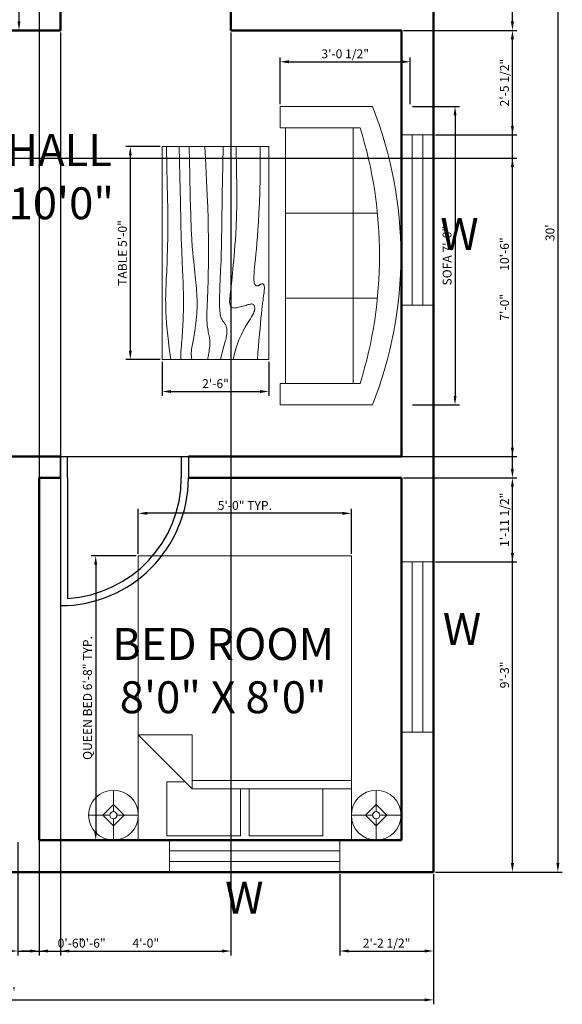
# Model space of a CAD drawing. Units: inches. Extents: x 2530 to 2846, y 1711 to 2145.
# Tile 2 of 3: x 2693 to 2846, y 1711 to 1989. Entities that reach past the tile are written whole.
import ezdxf

# ---------------------------------------------------------------- set-up
doc = ezdxf.new("R2010")
doc.units = ezdxf.units.IN
for name, color, linetype, lineweight in [('A-ANNO-DIMS', 2, 'Continuous', 18), ('A-ANNO-TEXT', 7, 'Continuous', 18), ('A-AREA-IDEN', 7, 'Continuous', 25), ('A-DOOR', 3, 'Continuous', 25), ('A-FURN', 8, 'Continuous', 18), ('A-GLAZ', 4, 'Continuous', 18), ('A-WALL', 7, 'Continuous', 50)]:
    doc.layers.add(name, color=color, linetype=linetype, lineweight=lineweight)
doc.styles.get("Standard").update_dxf_attribs({"font": 'arial.ttf'})
doc.dimstyles.new('ISO-25', dxfattribs={"dimtxt": 2.5, "dimasz": 2.5, "dimexe": 1.25, "dimexo": 0.625, "dimtad": 1, "dimdec": 0, "dimlunit": 3, "dimtxsty": 'Standard', "dimcen": 2.5, "dimadec": 0, "dimazin": 0, "dimtfac": 1, "dimtdec": 0, "dimtmove": 0, "dimatfit": 3, "dimfxl": 1, "dimarcsym": 0})

# ---------------------------------------------------------------- blocks, each defined once
blk = doc.blocks.new('Sofa - Roundback 7 ft.')
for p, q in [((-12.00002, -32.4421), (-12.00003, -6.5971)), ((11.99997, -32.4421), (11.99998, -6.5971)), ((-36.000027, -34), (-36.000027, -11.4696)), ((-35.999844, -13.3819), (35.9998, -13.3819)), ((35.99998, -34), (35.99998, -11.4696)), ((-36.000027, -32.4421), (35.99998, -32.4421))]:
    blk.add_line(p, q)
for points in [[(-36.000027, -34), (-42.000027, -34), (-42.000027, -8)], [(41.99998, -8), (41.99998, -34), (35.99998, -34)]]:
    blk.add_lwpolyline(points)
for centre, radius, start, end in [((0, -114.25), 114.25, 68.43141, 111.5686), ((-0.00001, -127.1968), 121.1968, 72.72033, 107.2797)]:
    blk.add_arc(centre, radius, start, end)
blk = doc.blocks.new('Table - Rectangular Woodgrain 60 x 30 in.')
for p, q in [((0, 0), (0, -30)), ((60, 0), (0, 0)), ((60, -30), (60, 0)), ((0, -30), (60, -30))]:
    blk.add_line(p, q)
for points in [[(0, -2.4), (4.8155, -2.418), (9.0302, -2.4688), (12.709, -2.5477), (15.9167, -2.65), (18.7181, -2.7711), (21.1781, -2.9063), (23.3616, -3.0508), (25.3333, -3.2), (27.1477, -3.3495), (28.8172, -3.4958), (30.3437, -3.636), (31.7291, -3.7667), (32.9756, -3.8849), (34.0849, -3.9875), (35.059, -4.0714), (35.9, -4.1334), (36.6114, -4.1711), (37.2041, -4.1854), (37.6906, -4.1779), (38.0833, -4.15), (38.3948, -4.1034), (38.6375, -4.0396), (38.8239, -3.9602), (38.9666, -3.8667), (39.0764, -3.7608), (39.1573, -3.6448), (39.2116, -3.521), (39.2416, -3.3917), (39.2498, -3.2593), (39.2385, -3.1261), (39.21, -2.9944), (39.1666, -2.8667), (39.111, -2.7447), (39.0468, -2.6281), (38.978, -2.5163), (38.9083, -2.4083), (38.8418, -2.3035), (38.7823, -2.201), (38.7337, -2.1001), (38.7, -2), (38.6844, -1.9003), (38.6875, -1.8021), (38.7094, -1.707), (38.75, -1.6167), (38.8094, -1.5326), (38.8875, -1.4563), (38.9844, -1.3893), (39.1, -1.3333), (39.2351, -1.2896), (39.3937, -1.2583), (39.5804, -1.2396), (39.8, -1.2333), (40.057, -1.2396), (40.3562, -1.2583), (40.7023, -1.2896), (41.1, -1.3333), (41.5547, -1.3895), (42.0755, -1.4573), (42.6721, -1.5361), (43.3542, -1.625), (44.1316, -1.7233), (45.014, -1.8302), (46.0114, -1.9449), (47.1333, -2.0667), (48.3862, -2.1947), (49.7625, -2.3281), (51.2513, -2.4663), (52.8416, -2.6083), (54.5226, -2.7535), (56.2833, -2.9011), (58.1127, -3.0501), (60, -3.2)], [(0, -9.2), (6.5759, -9.0858), (11.9385, -9.0365), (16.2527, -9.0418), (19.6833, -9.0917), (22.3952, -9.1759), (24.5531, -9.2844), (26.322, -9.4069), (27.8666, -9.5333), (29.3241, -9.6553), (30.7203, -9.7719), (32.0532, -9.8837), (33.3208, -9.9917), (34.5213, -10.0965), (35.6526, -10.199), (36.7128, -10.2999), (37.7, -10.4), (38.6129, -10.4996), (39.4531, -10.5969), (40.223, -10.6895), (40.925, -10.775), (41.5613, -10.8512), (42.1344, -10.9156), (42.6465, -10.966), (43.1, -11), (43.4976, -11.0158), (43.8437, -11.0136), (44.143, -10.9942), (44.4, -10.9583), (44.6195, -10.9069), (44.8062, -10.8406), (44.9648, -10.7603), (45.1, -10.6667), (45.2155, -10.5598), (45.3114, -10.4365), (45.3871, -10.2929), (45.4416, -10.125), (45.4743, -9.929), (45.4844, -9.7011), (45.4709, -9.4371), (45.4333, -9.1333), (45.3716, -8.7883), (45.2896, -8.4104), (45.1919, -8.0107), (45.0833, -7.6), (44.9685, -7.1893), (44.8521, -6.7896), (44.7388, -6.4117), (44.6333, -6.0667), (44.54, -5.7628), (44.4614, -5.4979), (44.4001, -5.2675), (44.3583, -5.0667), (44.3384, -4.8909), (44.3427, -4.7354), (44.3736, -4.5956), (44.4333, -4.4667), (44.5236, -4.3453), (44.6427, -4.2333), (44.7884, -4.1339), (44.9583, -4.05), (45.1501, -3.9849), (45.3614, -3.9417), (45.59, -3.9234), (45.8333, -3.9333), (46.0915, -3.9749), (46.3734, -4.0531), (46.6906, -4.1736), (47.0542, -4.3417), (47.4756, -4.5629), (47.9661, -4.8427), (48.5372, -5.1866), (49.2, -5.6), (49.9676, -6.0844), (50.8594, -6.625), (51.8965, -7.2031), (53.1, -7.8), (54.491, -8.3969), (56.0906, -8.975), (57.9199, -9.5156), (60, -10)], [(0, -12.8), (5.1847, -12.9322), (9.6213, -13.0323), (13.3963, -13.1059), (16.5958, -13.1583), (19.3063, -13.1952), (21.614, -13.2219), (23.6054, -13.2439), (25.3666, -13.2667), (26.9728, -13.2947), (28.4531, -13.3281), (29.8256, -13.3663), (31.1083, -13.4083), (32.3191, -13.4535), (33.476, -13.501), (34.597, -13.5501), (35.7, -13.6), (36.7984, -13.6497), (37.8875, -13.6979), (38.9578, -13.743), (40, -13.7833), (41.0047, -13.8174), (41.9625, -13.8438), (42.864, -13.8607), (43.7, -13.8667), (44.4631, -13.8604), (45.1552, -13.8417), (45.7801, -13.8104), (46.3416, -13.7667), (46.8439, -13.7104), (47.2906, -13.6417), (47.6858, -13.5604), (48.0333, -13.4667), (48.3375, -13.3608), (48.6042, -13.2448), (48.8396, -13.121), (49.05, -12.9917), (49.2417, -12.8593), (49.4208, -12.7261), (49.5937, -12.5944), (49.7667, -12.4667), (49.9452, -12.3451), (50.1323, -12.2313), (50.3303, -12.1268), (50.5416, -12.0333), (50.7686, -11.9524), (51.0135, -11.8854), (51.2788, -11.8341), (51.5666, -11.8), (51.8785, -11.7843), (52.2116, -11.7865), (52.562, -11.8059), (52.926, -11.8417), (53.2998, -11.8931), (53.6795, -11.9594), (54.0614, -12.0397), (54.4416, -12.1333), (54.8223, -12.2401), (55.2293, -12.3625), (55.6942, -12.5037), (56.2489, -12.6667), (56.9251, -12.8547), (57.7545, -13.0708), (58.7689, -13.3182), (60, -13.6)], [(0, -18), (5.124, -17.7273), (9.6609, -17.5057), (13.6705, -17.3303), (17.2125, -17.1958), (20.3467, -17.0973), (23.1328, -17.0297), (25.6307, -16.9878), (27.9, -16.9667), (29.9928, -16.9617), (31.9302, -16.9703), (33.7254, -16.9907), (35.3917, -17.0208), (36.9423, -17.0588), (38.3906, -17.1026), (39.7499, -17.1503), (41.0333, -17.2), (42.2519, -17.2496), (43.4073, -17.2969), (44.4986, -17.3395), (45.525, -17.375), (46.4858, -17.4012), (47.3802, -17.4156), (48.2074, -17.416), (48.9667, -17.4), (49.6583, -17.3662), (50.2872, -17.3167), (50.8595, -17.2547), (51.3812, -17.1833), (51.8584, -17.1057), (52.2971, -17.025), (52.7034, -16.9443), (53.0833, -16.8667), (53.443, -16.7951), (53.789, -16.7313), (54.128, -16.6768), (54.4666, -16.6334), (54.8115, -16.6024), (55.1693, -16.5854), (55.5465, -16.5841), (55.95, -16.6), (56.3828, -16.6337), (56.8346, -16.6823), (57.2915, -16.7418), (57.7396, -16.8084), (58.165, -16.878), (58.5539, -16.9469), (58.8924, -17.0111), (59.1666, -17.0667), (59.3679, -17.1107), (59.5078, -17.1438), (59.6032, -17.1675), (59.6708, -17.1833), (59.7275, -17.193), (59.7901, -17.1979), (59.8753, -17.1998), (60, -17.2)], [(0, -22.4), (8.0098, -22.2501), (14.4094, -22.1011), (19.4168, -21.9535), (23.25, -21.8083), (26.1269, -21.6663), (28.2656, -21.5281), (29.884, -21.3947), (31.2, -21.2667), (32.3967, -21.1448), (33.5172, -21.0292), (34.5697, -20.9198), (35.5625, -20.8167), (36.5037, -20.7198), (37.4015, -20.6292), (38.2642, -20.5448), (39.1, -20.4667), (39.9164, -20.3951), (40.7187, -20.3313), (41.5117, -20.2768), (42.3, -20.2333), (43.0883, -20.2024), (43.8812, -20.1854), (44.6836, -20.1841), (45.5, -20.2), (46.3328, -20.234), (47.1747, -20.2844), (48.0163, -20.3488), (48.8479, -20.425), (49.66, -20.5106), (50.4429, -20.6031), (51.1872, -20.7004), (51.8833, -20.8), (52.5246, -20.8999), (53.1166, -20.9995), (53.6681, -21.0983), (54.1875, -21.1958), (54.6834, -21.2919), (55.1646, -21.3859), (55.6394, -21.4777), (56.1167, -21.5667), (56.6028, -21.6515), (57.0961, -21.7266), (57.5929, -21.7852), (58.0896, -21.8208), (58.5823, -21.8268), (59.0674, -21.7964), (59.5412, -21.723), (60, -21.6)], [(0, -25.2), (8.6355, -25.0504), (15.7026, -24.9031), (21.4049, -24.7606), (25.9458, -24.625), (29.529, -24.4988), (32.3578, -24.3844), (34.6359, -24.284), (36.5667, -24.2), (38.3213, -24.1341), (39.9417, -24.0854), (41.437, -24.0523), (42.8167, -24.0333), (44.0901, -24.0268), (45.2667, -24.0313), (46.3557, -24.0451), (47.3667, -24.0667), (48.309, -24.0947), (49.1928, -24.1287), (50.0284, -24.168), (50.826, -24.2125), (51.5959, -24.2617), (52.3483, -24.3151), (53.0935, -24.3725), (53.8417, -24.4334), (54.6009, -24.497), (55.3699, -24.561), (56.1454, -24.6226), (56.9239, -24.6792), (57.7021, -24.7279), (58.4764, -24.7662), (59.2435, -24.7911), (60, -24.8)], [(0, -28.8), (5.6867, -28.6681), (10.45, -28.5698), (14.407, -28.5012), (17.675, -28.4584), (20.3711, -28.4374), (22.6125, -28.4344), (24.5164, -28.4455), (26.2, -28.4667), (27.762, -28.4947), (29.2276, -28.5281), (30.6033, -28.5663), (31.8958, -28.6084), (33.1118, -28.6535), (34.2578, -28.7011), (35.3405, -28.7501), (36.3666, -28.8), (37.3443, -28.8497), (38.288, -28.8974), (39.2137, -28.9412), (40.1375, -28.9792), (41.0753, -29.0093), (42.0432, -29.0297), (43.0572, -29.0384), (44.1333, -29.0333), (45.2936, -29.0114), (46.5843, -28.9641), (48.0579, -28.8816), (49.7666, -28.7542), (51.7629, -28.5721), (54.0989, -28.3255), (56.8272, -28.0048), (60, -27.6)]]:
    blk.add_lwpolyline(points)
blk = doc.blocks.new('Bed - Queen')
for p, q in [((0, -80.00003), (0, 0)), ((0, 0), (59.99999, 0)), ((59.99999, 0), (59.99999, -80.00003)), ((7.99999, -1.2), (28.79998, -1.2)), ((7.99999, -14.4), (7.99999, -1.2)), ((28.79998, -1.2), (28.79998, -14.4)), ((31.19999, -1.2), (51.99999, -1.2)), ((31.19999, -14.4), (31.19999, -1.2)), ((51.99999, -1.2), (51.99999, -16.4)), ((0, -14.4), (44.8, -14.4)), ((59.99999, -29.6), (44.8, -14.4)), ((44.8, -14.4), (44.8, -29.6)), ((51.99999, -16.4), (46.79936, -16.4)), ((44.8, -16.8), (0, -16.8)), ((44.8, -29.6), (59.99999, -29.6)), ((59.99999, -80.00003), (0, -80.00003))]:
    blk.add_line(p, q)
blk = doc.blocks.new('Lamp - Table')
for p, q in [((0, 7), (0, 1)), ((0, 3), (-3, 0)), ((3, 0), (0, 3)), ((-1, 0), (-7, 0)), ((-3, 0), (0, -3)), ((0, -3), (3, 0)), ((1, 0), (7, 0)), ((0, -1), (0, -7))]:
    blk.add_line(p, q)
for radius in [7, 1]:
    blk.add_circle((0, 0), radius)
blk = doc.blocks.new('*D12')
at = {"layer": 'A-ANNO-DIMS', "color": 0, "lineweight": -2, "transparency": 16777216}
for p, q in [((2810.07, 2108.63), (2845.75, 2108.63)), ((2844.5, 2106.13), (2844.5, 1751.13)), ((2810.07, 1748.63), (2845.75, 1748.63))]:
    blk.add_line(p, q, dxfattribs=at)
at = {"layer": 'A-ANNO-DIMS', "color": 0, "transparency": 16777216}
for points in [[(2844.08, 2106.13), (2844.91, 2106.13), (2844.5, 2108.63)], [(2844.08, 1751.13), (2844.91, 1751.13), (2844.5, 1748.63)]]:
    blk.add_solid(points, dxfattribs=at)
at = {"layer": 'Defpoints', "color": 0, "transparency": 16777216}
for p in [(2809.45, 2108.63), (2809.45, 1748.63), (2844.5, 1748.63)]:
    blk.add_point(p, dxfattribs=at)
at = {"layer": 'A-ANNO-DIMS', "color": 0, "transparency": 16777216, "insert": (2842.6, 1928.63), "char_height": 2.5, "attachment_point": 5, "rotation": 90}
blk.add_mtext("30'", dxfattribs=at)
blk = doc.blocks.new('*D14')
at = {"layer": 'A-ANNO-DIMS', "color": 0, "lineweight": -2, "transparency": 16777216}
for p, q in [((2569.45, 1748), (2569.45, 1711.38)), ((2809.45, 1748), (2809.45, 1711.38)), ((2571.95, 1712.63), (2806.95, 1712.63))]:
    blk.add_line(p, q, dxfattribs=at)
at = {"layer": 'A-ANNO-DIMS', "color": 0, "transparency": 16777216}
for points in [[(2571.95, 1713.05), (2571.95, 1712.21), (2569.45, 1712.63)], [(2806.95, 1713.05), (2806.95, 1712.21), (2809.45, 1712.63)]]:
    blk.add_solid(points, dxfattribs=at)
at = {"layer": 'Defpoints', "color": 0, "transparency": 16777216}
for p in [(2569.45, 1748.63), (2809.45, 1748.63), (2809.45, 1712.63)]:
    blk.add_point(p, dxfattribs=at)
at = {"layer": 'A-ANNO-DIMS', "color": 0, "transparency": 16777216, "insert": (2689.45, 1714.53), "char_height": 2.5, "attachment_point": 5}
blk.add_mtext("20'", dxfattribs=at)
blk = doc.blocks.new('WIN-48IN')
for p, q in [((0, 48), (0, 0)), ((9, 48), (0, 48)), ((3, 48), (3, 0)), ((6, 0), (6, 48)), ((9, 0), (9, 48)), ((0, 0), (9, 0))]:
    blk.add_line(p, q)
blk = doc.blocks.new('DOOR-SINGLE-36IN')
for p, q in [((0, 36), (0, 42)), ((2, 36), (2, 42)), ((34, 42), (34, 36)), ((36, 42), (36, 36)), ((0, 36), (0, 0)), ((2, 36), (2, 2.06))]:
    blk.add_line(p, q)
for radius, start in [(36, 270), (34, 273.3723)]:
    blk.add_arc((0, 36), radius, start, 0)
blk = doc.blocks.new('*D26')
at = {"layer": 'A-ANNO-DIMS', "color": 0, "lineweight": -2, "transparency": 16777216}
for p, q in [((2725.72, 1837.63), (2713.1, 1837.63)), ((2714.35, 1835.13), (2714.35, 1760.13)), ((2725.72, 1757.63), (2713.1, 1757.63))]:
    blk.add_line(p, q, dxfattribs=at)
at = {"layer": 'A-ANNO-DIMS', "color": 0, "transparency": 16777216}
for points in [[(2713.93, 1835.13), (2714.77, 1835.13), (2714.35, 1837.63)], [(2713.93, 1760.13), (2714.77, 1760.13), (2714.35, 1757.63)]]:
    blk.add_solid(points, dxfattribs=at)
at = {"layer": 'Defpoints', "color": 0, "transparency": 16777216}
for p in [(2726.35, 1837.63), (2714.35, 1757.63), (2726.35, 1757.63)]:
    blk.add_point(p, dxfattribs=at)
at = {"layer": 'A-ANNO-DIMS', "color": 0, "transparency": 16777216, "insert": (2712.36, 1797.63), "char_height": 2.5, "attachment_point": 5, "rotation": 90}
blk.add_mtext('QUEEN BED 6\'-8" TYP.', dxfattribs=at)
blk = doc.blocks.new('*D27')
at = {"layer": 'A-ANNO-DIMS', "color": 0, "lineweight": -2, "transparency": 16777216}
for p, q in [((2726.35, 1838.25), (2726.35, 1850.88)), ((2783.85, 1849.63), (2728.85, 1849.63)), ((2786.35, 1838.25), (2786.35, 1850.88))]:
    blk.add_line(p, q, dxfattribs=at)
at = {"layer": 'A-ANNO-DIMS', "color": 0, "transparency": 16777216}
for points in [[(2728.85, 1850.05), (2728.85, 1849.21), (2726.35, 1849.63)], [(2783.85, 1850.05), (2783.85, 1849.21), (2786.35, 1849.63)]]:
    blk.add_solid(points, dxfattribs=at)
at = {"layer": 'Defpoints', "color": 0, "transparency": 16777216}
for p in [(2726.35, 1849.63), (2726.35, 1837.63), (2786.35, 1837.63)]:
    blk.add_point(p, dxfattribs=at)
at = {"layer": 'A-ANNO-DIMS', "color": 0, "transparency": 16777216, "insert": (2756.35, 1851.53), "char_height": 2.5, "attachment_point": 5}
blk.add_mtext('5\'-0" TYP.', dxfattribs=at)
blk = doc.blocks.new('*D32')
at = {"layer": 'A-ANNO-DIMS', "color": 0, "lineweight": -2, "transparency": 16777216}
for p, q in [((2687.07, 2027.63), (2694, 2027.63)), ((2692.75, 2025.13), (2692.75, 1988.13)), ((2687.07, 1985.63), (2694, 1985.63))]:
    blk.add_line(p, q, dxfattribs=at)
at = {"layer": 'A-ANNO-DIMS', "color": 0, "transparency": 16777216}
for points in [[(2692.33, 2025.13), (2693.17, 2025.13), (2692.75, 2027.63)], [(2692.33, 1988.13), (2693.17, 1988.13), (2692.75, 1985.63)]]:
    blk.add_solid(points, dxfattribs=at)
at = {"layer": 'Defpoints', "color": 0, "transparency": 16777216}
for p in [(2686.45, 2027.63), (2686.45, 1985.63), (2692.75, 1985.63)]:
    blk.add_point(p, dxfattribs=at)
at = {"layer": 'A-ANNO-DIMS', "color": 0, "transparency": 16777216, "insert": (2690.83, 2006.63), "char_height": 2.5, "attachment_point": 5, "rotation": 90}
blk.add_mtext('DOOR 3\'-6" TYP.', dxfattribs=at)
blk = doc.blocks.new('*D36')
at = {"layer": 'A-ANNO-DIMS', "color": 0, "lineweight": -2, "transparency": 16777216}
for p, q in [((2803.57, 1964.18), (2816.79, 1964.18)), ((2815.54, 1961.68), (2815.54, 1882.68)), ((2803.57, 1880.18), (2816.79, 1880.18))]:
    blk.add_line(p, q, dxfattribs=at)
at = {"layer": 'A-ANNO-DIMS', "color": 0, "transparency": 16777216}
for points in [[(2815.13, 1961.68), (2815.96, 1961.68), (2815.54, 1964.18)], [(2815.13, 1882.68), (2815.96, 1882.68), (2815.54, 1880.18)]]:
    blk.add_solid(points, dxfattribs=at)
at = {"layer": 'Defpoints', "color": 0, "transparency": 16777216}
for p in [(2802.94, 1964.18), (2802.94, 1880.18), (2815.54, 1880.18)]:
    blk.add_point(p, dxfattribs=at)
at = {"layer": 'A-ANNO-DIMS', "color": 0, "transparency": 16777216, "insert": (2813.62, 1922.18), "char_height": 2.5, "attachment_point": 5, "rotation": 90}
blk.add_mtext('SOFA 7\'-0"', dxfattribs=at)
blk = doc.blocks.new('*D37')
at = {"layer": 'A-ANNO-DIMS', "color": 0, "lineweight": -2, "transparency": 16777216}
for p, q in [((2766.28, 1964.8), (2766.28, 1978.03)), ((2802.94, 1964.8), (2802.94, 1978.03)), ((2768.78, 1976.78), (2800.44, 1976.78))]:
    blk.add_line(p, q, dxfattribs=at)
at = {"layer": 'A-ANNO-DIMS', "color": 0, "transparency": 16777216}
for points in [[(2768.78, 1977.2), (2768.78, 1976.36), (2766.28, 1976.78)], [(2800.44, 1977.2), (2800.44, 1976.36), (2802.94, 1976.78)]]:
    blk.add_solid(points, dxfattribs=at)
at = {"layer": 'Defpoints', "color": 0, "transparency": 16777216}
for p in [(2802.94, 1976.78), (2766.28, 1964.18), (2802.94, 1964.18)]:
    blk.add_point(p, dxfattribs=at)
at = {"layer": 'A-ANNO-DIMS', "color": 0, "transparency": 16777216, "insert": (2784.61, 1978.7), "char_height": 2.5, "attachment_point": 5}
blk.add_mtext('3\'-0 1/2"', dxfattribs=at)
blk = doc.blocks.new('*D38')
at = {"layer": 'A-ANNO-DIMS', "color": 0, "lineweight": -2, "transparency": 16777216}
for p, q in [((2732.47, 1952.93), (2722.84, 1952.93)), ((2724.09, 1950.43), (2724.09, 1895.43)), ((2732.47, 1892.93), (2722.84, 1892.93))]:
    blk.add_line(p, q, dxfattribs=at)
at = {"layer": 'A-ANNO-DIMS', "color": 0, "transparency": 16777216}
for points in [[(2723.68, 1950.43), (2724.51, 1950.43), (2724.09, 1952.93)], [(2723.68, 1895.43), (2724.51, 1895.43), (2724.09, 1892.93)]]:
    blk.add_solid(points, dxfattribs=at)
at = {"layer": 'Defpoints', "color": 0, "transparency": 16777216}
for p in [(2733.09, 1952.93), (2724.09, 1892.93), (2733.09, 1892.93)]:
    blk.add_point(p, dxfattribs=at)
at = {"layer": 'A-ANNO-DIMS', "color": 0, "transparency": 16777216, "insert": (2722.19, 1922.93), "char_height": 2.5, "attachment_point": 5, "rotation": 90}
blk.add_mtext('TABLE 5\'-0"', dxfattribs=at)
blk = doc.blocks.new('*D39')
at = {"layer": 'A-ANNO-DIMS', "color": 0, "lineweight": -2, "transparency": 16777216}
for p, q in [((2733.09, 1892.3), (2733.09, 1882.68)), ((2763.09, 1892.3), (2763.09, 1882.68)), ((2735.59, 1883.93), (2760.59, 1883.93))]:
    blk.add_line(p, q, dxfattribs=at)
at = {"layer": 'A-ANNO-DIMS', "color": 0, "transparency": 16777216}
for points in [[(2735.59, 1884.34), (2735.59, 1883.51), (2733.09, 1883.93)], [(2760.59, 1884.34), (2760.59, 1883.51), (2763.09, 1883.93)]]:
    blk.add_solid(points, dxfattribs=at)
at = {"layer": 'Defpoints', "color": 0, "transparency": 16777216}
for p in [(2733.09, 1892.93), (2763.09, 1892.93), (2763.09, 1883.93)]:
    blk.add_point(p, dxfattribs=at)
at = {"layer": 'A-ANNO-DIMS', "color": 0, "transparency": 16777216, "insert": (2748.09, 1885.83), "char_height": 2.5, "attachment_point": 5}
blk.add_mtext('2\'-6"', dxfattribs=at)
blk = doc.blocks.new('*D52')
at = {"layer": 'A-ANNO-DIMS', "color": 0, "lineweight": -2, "transparency": 16777216}
for p, q in [((2704.45, 1985), (2704.45, 1725.13)), ((2752.45, 1985), (2752.45, 1725.13)), ((2706.95, 1726.38), (2749.95, 1726.38))]:
    blk.add_line(p, q, dxfattribs=at)
at = {"layer": 'A-ANNO-DIMS', "color": 0, "transparency": 16777216}
for points in [[(2706.95, 1726.8), (2706.95, 1725.96), (2704.45, 1726.38)], [(2749.95, 1726.8), (2749.95, 1725.96), (2752.45, 1726.38)]]:
    blk.add_solid(points, dxfattribs=at)
at = {"layer": 'Defpoints', "color": 0, "transparency": 16777216}
for p in [(2704.45, 1985.63), (2752.45, 1985.63), (2752.45, 1726.38)]:
    blk.add_point(p, dxfattribs=at)
at = {"layer": 'A-ANNO-DIMS', "color": 0, "transparency": 16777216, "insert": (2728.45, 1728.28), "char_height": 2.5, "attachment_point": 5}
blk.add_mtext('4\'-0"', dxfattribs=at)
blk = doc.blocks.new('*D53')
at = {"layer": 'A-ANNO-DIMS', "color": 0, "lineweight": -2, "transparency": 16777216}
for p, q in [((2801.07, 1859.63), (2832.95, 1859.63)), ((2831.7, 1751.13), (2831.7, 1857.13)), ((2810.07, 1748.63), (2832.95, 1748.63))]:
    blk.add_line(p, q, dxfattribs=at)
at = {"layer": 'A-ANNO-DIMS', "color": 0, "transparency": 16777216}
for points in [[(2831.28, 1857.13), (2832.12, 1857.13), (2831.7, 1859.63)], [(2831.28, 1751.13), (2832.12, 1751.13), (2831.7, 1748.63)]]:
    blk.add_solid(points, dxfattribs=at)
at = {"layer": 'Defpoints', "color": 0, "transparency": 16777216}
for p in [(2800.45, 1859.63), (2831.7, 1859.63), (2809.45, 1748.63)]:
    blk.add_point(p, dxfattribs=at)
at = {"layer": 'A-ANNO-DIMS', "color": 0, "transparency": 16777216, "insert": (2829.8, 1804.13), "char_height": 2.5, "attachment_point": 5, "rotation": 90}
blk.add_mtext('9\'-3"', dxfattribs=at)
blk = doc.blocks.new('*D54')
at = {"layer": 'A-ANNO-DIMS', "color": 0, "lineweight": -2, "transparency": 16777216}
for p, q in [((2801.07, 1985.63), (2832.95, 1985.63)), ((2831.7, 1862.13), (2831.7, 1983.13)), ((2801.07, 1859.63), (2832.95, 1859.63))]:
    blk.add_line(p, q, dxfattribs=at)
at = {"layer": 'A-ANNO-DIMS', "color": 0, "transparency": 16777216}
for points in [[(2831.28, 1983.13), (2832.12, 1983.13), (2831.7, 1985.63)], [(2831.28, 1862.13), (2832.12, 1862.13), (2831.7, 1859.63)]]:
    blk.add_solid(points, dxfattribs=at)
at = {"layer": 'Defpoints', "color": 0, "transparency": 16777216}
for p in [(2800.45, 1985.63), (2831.7, 1985.63), (2800.45, 1859.63)]:
    blk.add_point(p, dxfattribs=at)
at = {"layer": 'A-ANNO-DIMS', "color": 0, "transparency": 16777216, "insert": (2829.8, 1922.63), "char_height": 2.5, "attachment_point": 5, "rotation": 90}
blk.add_mtext('10\'-6"', dxfattribs=at)
blk = doc.blocks.new('*D55')
at = {"layer": 'A-ANNO-DIMS', "color": 0, "lineweight": -2, "transparency": 16777216}
for p, q in [((2801.07, 2051.63), (2832.95, 2051.63)), ((2831.7, 1988.13), (2831.7, 2049.13)), ((2801.07, 1985.63), (2832.95, 1985.63))]:
    blk.add_line(p, q, dxfattribs=at)
at = {"layer": 'A-ANNO-DIMS', "color": 0, "transparency": 16777216}
for points in [[(2831.28, 2049.13), (2832.12, 2049.13), (2831.7, 2051.63)], [(2831.28, 1988.13), (2832.12, 1988.13), (2831.7, 1985.63)]]:
    blk.add_solid(points, dxfattribs=at)
at = {"layer": 'Defpoints', "color": 0, "transparency": 16777216}
for p in [(2800.45, 2051.63), (2831.7, 2051.63), (2800.45, 1985.63)]:
    blk.add_point(p, dxfattribs=at)
at = {"layer": 'A-ANNO-DIMS', "color": 0, "transparency": 16777216, "insert": (2829.8, 2018.63), "char_height": 2.5, "attachment_point": 5, "rotation": 90}
blk.add_mtext('5\'-6"', dxfattribs=at)
blk = doc.blocks.new('*D57')
at = {"layer": 'A-ANNO-DIMS', "color": 0, "lineweight": -2, "transparency": 16777216}
for p, q in [((2692.45, 1757), (2692.45, 1725.13)), ((2698.45, 1757), (2698.45, 1725.13)), ((2689.95, 1726.38), (2687.45, 1726.38)), ((2692.45, 1726.38), (2698.45, 1726.38)), ((2700.95, 1726.38), (2711.34, 1726.38))]:
    blk.add_line(p, q, dxfattribs=at)
at = {"layer": 'A-ANNO-DIMS', "color": 0, "transparency": 16777216}
for points in [[(2689.95, 1726.8), (2689.95, 1725.96), (2692.45, 1726.38)], [(2700.95, 1726.8), (2700.95, 1725.96), (2698.45, 1726.38)]]:
    blk.add_solid(points, dxfattribs=at)
at = {"layer": 'Defpoints', "color": 0, "transparency": 16777216}
for p in [(2692.45, 1757.63), (2698.45, 1757.63), (2698.45, 1726.38)]:
    blk.add_point(p, dxfattribs=at)
at = {"layer": 'A-ANNO-DIMS', "color": 0, "transparency": 16777216, "insert": (2707.4, 1728.28), "char_height": 2.5, "attachment_point": 5}
blk.add_mtext('0\'-6"', dxfattribs=at)
blk = doc.blocks.new('*D58')
at = {"layer": 'A-ANNO-DIMS', "color": 0, "lineweight": -2, "transparency": 16777216}
for p, q in [((2627.07, 1949.63), (2832.95, 1949.63)), ((2831.7, 1868.13), (2831.7, 1947.13)), ((2627.07, 1865.63), (2832.95, 1865.63))]:
    blk.add_line(p, q, dxfattribs=at)
at = {"layer": 'A-ANNO-DIMS', "color": 0, "transparency": 16777216}
for points in [[(2831.28, 1947.13), (2832.12, 1947.13), (2831.7, 1949.63)], [(2831.28, 1868.13), (2832.12, 1868.13), (2831.7, 1865.63)]]:
    blk.add_solid(points, dxfattribs=at)
at = {"layer": 'Defpoints', "color": 0, "transparency": 16777216}
for p in [(2626.45, 1949.63), (2831.7, 1949.63), (2626.45, 1865.63)]:
    blk.add_point(p, dxfattribs=at)
at = {"layer": 'A-ANNO-DIMS', "color": 0, "transparency": 16777216, "insert": (2829.8, 1907.63), "char_height": 2.5, "attachment_point": 5, "rotation": 90}
blk.add_mtext('7\'-0"', dxfattribs=at)
blk = doc.blocks.new('*D61')
at = {"layer": 'A-ANNO-DIMS', "color": 0, "lineweight": -2, "transparency": 16777216}
for p, q in [((2783.09, 1748), (2783.09, 1725.13)), ((2809.45, 1748), (2809.45, 1725.13)), ((2785.59, 1726.38), (2806.95, 1726.38))]:
    blk.add_line(p, q, dxfattribs=at)
at = {"layer": 'A-ANNO-DIMS', "color": 0, "transparency": 16777216}
for points in [[(2785.59, 1726.8), (2785.59, 1725.96), (2783.09, 1726.38)], [(2806.95, 1726.8), (2806.95, 1725.96), (2809.45, 1726.38)]]:
    blk.add_solid(points, dxfattribs=at)
at = {"layer": 'Defpoints', "color": 0, "transparency": 16777216}
for p in [(2783.09, 1748.63), (2809.45, 1748.63), (2809.45, 1726.38)]:
    blk.add_point(p, dxfattribs=at)
at = {"layer": 'A-ANNO-DIMS', "color": 0, "transparency": 16777216, "insert": (2796.27, 1728.3), "char_height": 2.5, "attachment_point": 5}
blk.add_mtext('2\'-2 1/2"', dxfattribs=at)
blk = doc.blocks.new('*D65')
at = {"layer": 'A-ANNO-DIMS', "color": 0, "lineweight": -2, "transparency": 16777216}
for p, q in [((2801.07, 1859.63), (2832.95, 1859.63)), ((2831.7, 1838.49), (2831.7, 1857.13)), ((2810.07, 1835.99), (2832.95, 1835.99))]:
    blk.add_line(p, q, dxfattribs=at)
at = {"layer": 'A-ANNO-DIMS', "color": 0, "transparency": 16777216}
for points in [[(2831.28, 1857.13), (2832.12, 1857.13), (2831.7, 1859.63)], [(2831.28, 1838.49), (2832.12, 1838.49), (2831.7, 1835.99)]]:
    blk.add_solid(points, dxfattribs=at)
at = {"layer": 'Defpoints', "color": 0, "transparency": 16777216}
for p in [(2800.45, 1859.63), (2831.7, 1859.63), (2809.45, 1835.99)]:
    blk.add_point(p, dxfattribs=at)
at = {"layer": 'A-ANNO-DIMS', "color": 0, "transparency": 16777216, "insert": (2829.78, 1847.81), "char_height": 2.5, "attachment_point": 5, "rotation": 90}
blk.add_mtext('1\'-11 1/2"', dxfattribs=at)
blk = doc.blocks.new('*D66')
at = {"layer": 'A-ANNO-DIMS', "color": 0, "lineweight": -2, "transparency": 16777216}
for p, q in [((2801.07, 1985.63), (2832.95, 1985.63)), ((2831.7, 1958.7), (2831.7, 1983.13)), ((2810.07, 1956.2), (2832.95, 1956.2))]:
    blk.add_line(p, q, dxfattribs=at)
at = {"layer": 'A-ANNO-DIMS', "color": 0, "transparency": 16777216}
for points in [[(2831.28, 1983.13), (2832.12, 1983.13), (2831.7, 1985.63)], [(2831.28, 1958.7), (2832.12, 1958.7), (2831.7, 1956.2)]]:
    blk.add_solid(points, dxfattribs=at)
at = {"layer": 'Defpoints', "color": 0, "transparency": 16777216}
for p in [(2800.45, 1985.63), (2831.7, 1985.63), (2809.45, 1956.2)]:
    blk.add_point(p, dxfattribs=at)
at = {"layer": 'A-ANNO-DIMS', "color": 0, "transparency": 16777216, "insert": (2829.78, 1970.91), "char_height": 2.5, "attachment_point": 5, "rotation": 90}
blk.add_mtext('2\'-5 1/2"', dxfattribs=at)
blk = doc.blocks.new('*D72')
at = {"layer": 'A-ANNO-DIMS', "color": 0, "lineweight": -2, "transparency": 16777216}
for p, q in [((2698.45, 1991), (2698.45, 1725.13)), ((2704.45, 1985), (2704.45, 1725.13)), ((2695.95, 1726.38), (2693.45, 1726.38)), ((2698.45, 1726.38), (2704.45, 1726.38)), ((2706.95, 1726.38), (2717.34, 1726.38))]:
    blk.add_line(p, q, dxfattribs=at)
at = {"layer": 'A-ANNO-DIMS', "color": 0, "transparency": 16777216}
for points in [[(2695.95, 1726.8), (2695.95, 1725.96), (2698.45, 1726.38)], [(2706.95, 1726.8), (2706.95, 1725.96), (2704.45, 1726.38)]]:
    blk.add_solid(points, dxfattribs=at)
at = {"layer": 'Defpoints', "color": 0, "transparency": 16777216}
for p in [(2698.45, 1991.63), (2704.45, 1985.63), (2704.45, 1726.38)]:
    blk.add_point(p, dxfattribs=at)
at = {"layer": 'A-ANNO-DIMS', "color": 0, "transparency": 16777216, "insert": (2713.4, 1728.28), "char_height": 2.5, "attachment_point": 5}
blk.add_mtext('0\'-6"', dxfattribs=at)

msp = doc.modelspace()

# ---------------------------------------------------------------- linework, layer by layer
at = {"layer": 'A-WALL'}
for p, q in [((2809.45, 2108.63), (2809.45, 1748.63)), ((2704.45, 1991.63), (2704.45, 1985.63)), ((2752.45, 1985.63), (2752.45, 1991.63)), ((2686.45, 1985.63), (2704.45, 1985.63)), ((2752.45, 1985.63), (2800.45, 1985.63)), ((2800.45, 1985.63), (2800.45, 1865.63)), ((2680.45, 1865.63), (2704.45, 1865.63)), ((2740.45, 1865.63), (2800.45, 1865.63)), ((2698.45, 1859.63), (2698.45, 1757.63)), ((2698.45, 1859.63), (2704.45, 1859.63)), ((2698.45, 1859.63), (2704.45, 1859.63)), ((2740.45, 1859.63), (2800.45, 1859.63)), ((2800.45, 1859.63), (2800.45, 1757.63)), ((2800.45, 1757.63), (2698.45, 1757.63)), ((2809.45, 1748.63), (2680.45, 1748.63))]:
    msp.add_line(p, q, dxfattribs=at)

# ---------------------------------------------------------------- block references
at = {"layer": 'A-DOOR'}
msp.add_blockref('DOOR-SINGLE-36IN', (2704.45, 1823.63), dxfattribs=at)
at = {"layer": 'A-FURN'}
for name, p, rotation in [('Sofa - Roundback 7 ft.', (2800.28, 1922.18), 270), ('Table - Rectangular Woodgrain 60 x 30 in.', (2763.09, 1952.93), 270), ('Bed - Queen', (2786.35, 1757.63), 180), ('Lamp - Table', (2719.35, 1764.63), 180), ('Lamp - Table', (2793.35, 1764.63), 180)]:
    msp.add_blockref(name, p, dxfattribs=dict(at, rotation=rotation))
at = {"layer": 'A-GLAZ'}
for p, rotation in [((2809.45, 1956.2), 180), ((2809.45, 1835.99), 180), ((2783.09, 1748.63), 90.00000000000045)]:
    msp.add_blockref('WIN-48IN', p, dxfattribs=dict(at, rotation=rotation))

# ---------------------------------------------------------------- texts
at = {"layer": 'A-ANNO-TEXT', "char_height": 9, "attachment_point": 1}
for insert in [(2785.63, 1932.81), (2786.35, 1821.55), (2725.04, 1745.88)]:
    msp.add_mtext_dynamic_manual_height_columns('\\pxqc;W', width=62.3253, gutter_width=12.5, heights=[0], dxfattribs=dict(at, insert=insert))
at = {"layer": 'A-AREA-IDEN', "char_height": 9, "attachment_point": 1}
for s, insert in [('\\pxqc;LIVING HALL\\P14\'6" X 10\'0"', (2639.57, 1956.44)), ('\\pxqc;BED ROOM \\P8\'0" X 8\'0"', (2706.26, 1817.34))]:
    msp.add_mtext_dynamic_manual_height_columns(s, width=87.9878, gutter_width=12.5, heights=[0], dxfattribs=dict(at, insert=insert))

# ---------------------------------------------------------------- dimensions: what is measured, and where the dimension line sits
at = {"layer": 'A-ANNO-DIMS'}
for base, p1, p2, override, picture, middle in [((2844.5, 1748.63), (2809.45, 2108.63), (2809.45, 1748.63), {"dimclrd": 0, "dimclre": 0, "dimclrt": 0}, '*D12', (2842.6, 1928.63)), ((2831.7, 2051.63), (2800.45, 1985.63), (2800.45, 2051.63), {"dimdec": 1, "dimlfac": 1, "dimrnd": 0, "dimzin": 1, "dimdsep": 46, "dimlunit": 4, "dimfrac": 2}, '*D55', (2829.8, 2018.63)), ((2831.7, 1985.63), (2800.45, 1859.63), (2800.45, 1985.63), {"dimdec": 1, "dimlfac": 1, "dimrnd": 0, "dimzin": 1, "dimdsep": 46, "dimlunit": 4, "dimfrac": 2}, '*D54', (2829.8, 1922.63)), ((2831.7, 1985.63), (2809.45, 1956.2), (2800.45, 1985.63), {"dimdec": 1, "dimlfac": 1, "dimrnd": 0, "dimzin": 1, "dimdsep": 46, "dimlunit": 4, "dimfrac": 2}, '*D66', (2829.78, 1970.91)), ((2831.7, 1949.63), (2626.45, 1865.63), (2626.45, 1949.63), {"dimdec": 1, "dimlfac": 1, "dimrnd": 0, "dimzin": 1, "dimdsep": 46, "dimlunit": 4, "dimfrac": 2}, '*D58', (2829.8, 1907.63)), ((2831.7, 1859.63), (2809.45, 1748.63), (2800.45, 1859.63), {"dimdec": 1, "dimlfac": 1, "dimrnd": 0, "dimzin": 1, "dimdsep": 46, "dimlunit": 4, "dimfrac": 2}, '*D53', (2829.8, 1804.13)), ((2831.7, 1859.63), (2809.45, 1835.99), (2800.45, 1859.63), {"dimdec": 1, "dimlfac": 1, "dimrnd": 0, "dimzin": 1, "dimdsep": 46, "dimlunit": 4, "dimfrac": 2}, '*D65', (2829.78, 1847.81))]:
    dim = msp.add_linear_dim(base=base, p1=p1, p2=p2, angle=90, dimstyle='ISO-25', override=override, dxfattribs=at)
    dim.commit()
    dim.dimension.update_dxf_attribs({"geometry": picture, "text_midpoint": middle})
for base, p1, p2, angle, text, picture, middle in [((2692.75, 1985.63), (2686.45, 2027.63), (2686.45, 1985.63), 270, 'DOOR <> TYP.', '*D32', (2690.83, 2006.63)), ((2815.54, 1880.18), (2802.94, 1964.18), (2802.94, 1880.18), 270, 'SOFA <>', '*D36', (2813.62, 1922.18)), ((2724.09, 1892.93), (2733.09, 1952.93), (2733.09, 1892.93), 270, 'TABLE <>', '*D38', (2722.19, 1922.93)), ((2726.35, 1849.63), (2786.35, 1837.63), (2726.35, 1837.63), 180, '<> TYP.', '*D27', (2756.35, 1851.53)), ((2714.35, 1757.63), (2726.35, 1837.63), (2726.35, 1757.63), 270, 'QUEEN BED <> TYP.', '*D26', (2712.36, 1797.63))]:
    dim = msp.add_linear_dim(base=base, p1=p1, p2=p2, angle=angle, text=text, dimstyle='ISO-25', override={"dimdec": 1, "dimlfac": 1, "dimrnd": 0, "dimzin": 1, "dimdsep": 46, "dimlunit": 4, "dimfrac": 2}, dxfattribs=at)
    dim.commit()
    dim.dimension.update_dxf_attribs({"geometry": picture, "text_midpoint": middle})
for base, p1, p2, override, picture, middle in [((2704.45, 1726.38), (2698.45, 1991.63), (2704.45, 1985.63), {"dimdec": 1, "dimlfac": 1, "dimrnd": 0, "dimzin": 1, "dimdsep": 46, "dimlunit": 4, "dimfrac": 2}, '*D72', (2713.4, 1728.28)), ((2752.45, 1726.38), (2704.45, 1985.63), (2752.45, 1985.63), {"dimdec": 1, "dimlfac": 1, "dimrnd": 0, "dimzin": 1, "dimdsep": 46, "dimlunit": 4, "dimfrac": 2}, '*D52', (2728.45, 1728.28)), ((2802.94, 1976.78), (2766.28, 1964.18), (2802.94, 1964.18), {"dimdec": 1, "dimlfac": 1, "dimrnd": 0, "dimzin": 1, "dimdsep": 46, "dimlunit": 4, "dimfrac": 2}, '*D37', (2784.61, 1978.7)), ((2763.09, 1883.93), (2733.09, 1892.93), (2763.09, 1892.93), {"dimdec": 1, "dimlfac": 1, "dimrnd": 0, "dimzin": 1, "dimdsep": 46, "dimlunit": 4, "dimfrac": 2}, '*D39', (2748.09, 1885.83)), ((2698.45, 1726.38), (2692.45, 1757.63), (2698.45, 1757.63), {"dimdec": 1, "dimlfac": 1, "dimrnd": 0, "dimzin": 1, "dimdsep": 46, "dimlunit": 4, "dimfrac": 2}, '*D57', (2707.4, 1728.28)), ((2809.45, 1712.63), (2569.45, 1748.63), (2809.45, 1748.63), {"dimclrd": 0, "dimclre": 0, "dimclrt": 0}, '*D14', (2689.45, 1714.53)), ((2809.45, 1726.38), (2783.09, 1748.63), (2809.45, 1748.63), {"dimdec": 1, "dimlfac": 1, "dimrnd": 0, "dimzin": 1, "dimdsep": 46, "dimlunit": 4, "dimfrac": 2}, '*D61', (2796.27, 1728.3))]:
    dim = msp.add_linear_dim(base=base, p1=p1, p2=p2, dimstyle='ISO-25', override=override, dxfattribs=at)
    dim.commit()
    dim.dimension.update_dxf_attribs({"geometry": picture, "text_midpoint": middle})

doc.saveas('drawing.dxf')
